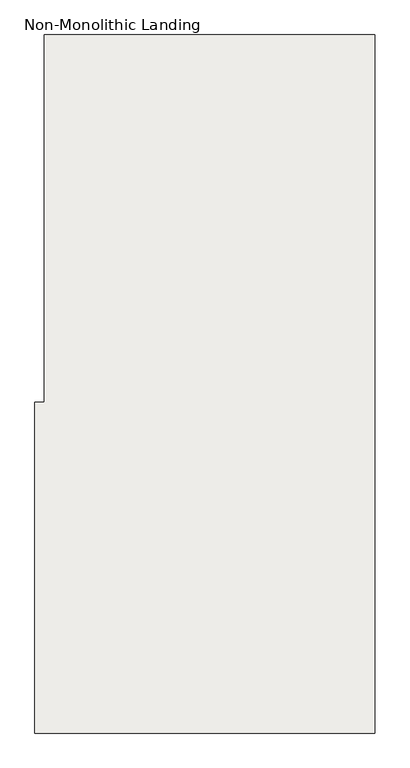
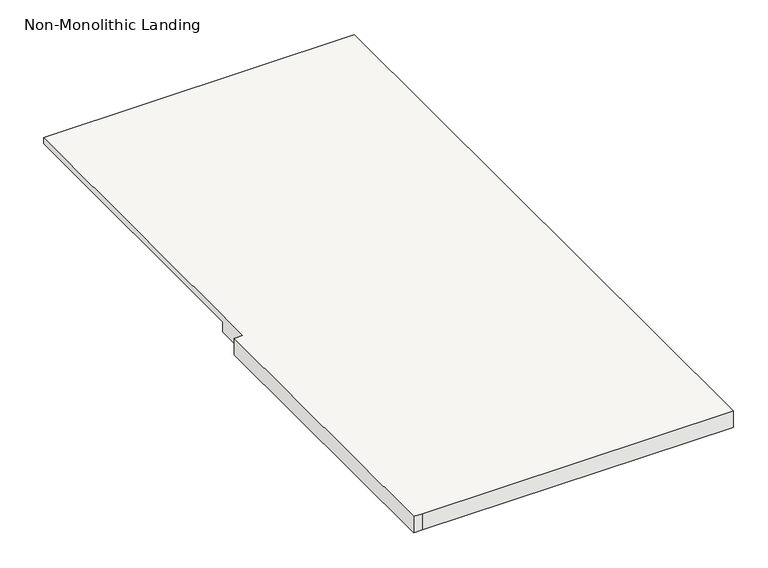
"""IFC4 building model written with IfcOpenShell, lengths in millimetres: slab geometry, Non-Monolithic Landing."""

from ifc_helpers import new_model, si_unit, origin, place, context, project, spatial, faceted_brep, source, transform, mapped, element, save


def non_monolithic_landing_8fd7ddd1(model_context):
    return source(origin(), model_context, "Body", "Brep", [
        faceted_brep([(923.4845537, -3822.9544725, 23983.95), (948.8845537, -3822.9544725, 23958.55), (948.8845537, -4737.3544725, 23958.55), (923.4845537, -4737.3544725, 23983.95), (923.4845537, -4838.9544725, 24003.0), (898.0845537, -4838.9544725, 24003.0), (898.0845537, -5753.3544725, 24003.0), (923.4845537, -5753.3544725, 24003.0), (1837.8845537, -5753.3544725, 24003.0), (1837.8845537, -3822.9544725, 24003.0), (923.4845537, -3822.9544725, 24003.0), (948.8845537, -4737.3544725, 23952.2), (948.8845537, -3822.9544725, 23952.2), (1837.8845537, -3822.9544725, 23952.2), (1837.8845537, -5753.3544725, 23952.2), (923.4845537, -5753.3544725, 23952.2), (898.0845537, -5753.3544725, 23952.2), (898.0845537, -4838.9544725, 23952.2), (923.4845537, -4838.9544725, 23952.2), (923.4845537, -4737.3544725, 23952.2)], [[[0, 1, 2, 3]], [[4, 5, 6, 7, 8, 9, 10]], [[11, 12, 13, 14, 15, 16, 17, 18, 19]], [[12, 11, 2, 1]], [[11, 19, 3, 2]], [[4, 10, 0, 3, 19, 18]], [[5, 4, 18, 17]], [[6, 5, 17, 16]], [[7, 6, 16, 15]], [[8, 7, 15, 14]], [[9, 8, 14, 13]], [[10, 9, 13, 12, 1, 0]]]),
    ])


if __name__ == "__main__":
    model = new_model("IFC4")
    model_context = context("Model", 3, world=origin())
    ifc_project = project(units=[si_unit("LENGTHUNIT", "METRE", prefix="MILLI")], contexts=[model_context])
    site = spatial("IfcSite", under=ifc_project)
    building = spatial("IfcBuilding", under=site)
    placement = place(None, origin())
    non_monolithic_landing_shape = non_monolithic_landing_8fd7ddd1(model_context)
    element("IfcSlab", 1, ObjectType="Non-Monolithic Landing", at=placement, inside=building, context=model_context, shape_type="MappedRepresentation", body=[
        mapped(non_monolithic_landing_shape, transform((0.0, 0.0, 0.0), x_axis=(1.0, 0.0, 0.0), y_axis=(0.0, 1.0, 0.0), z_axis=(0.0, 0.0, 1.0))),
    ])
    save(model, "model.ifc")
